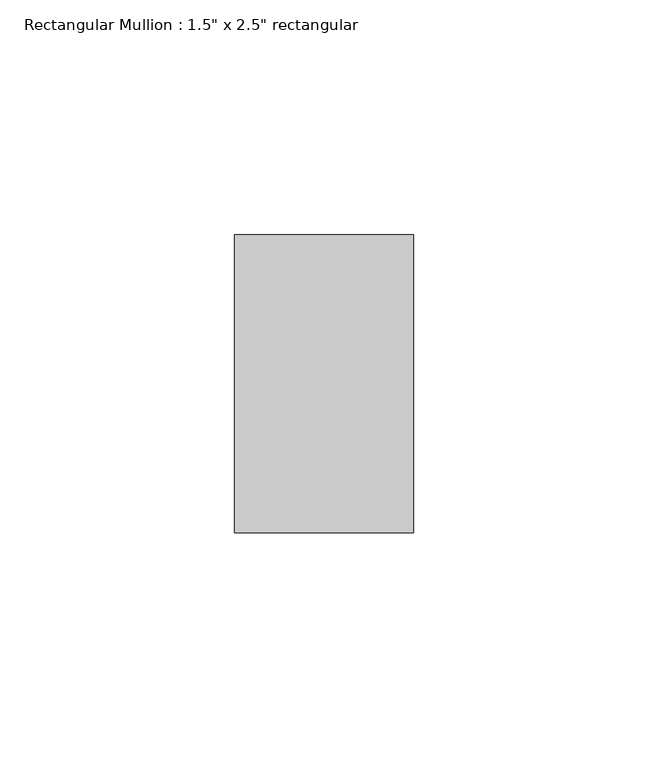
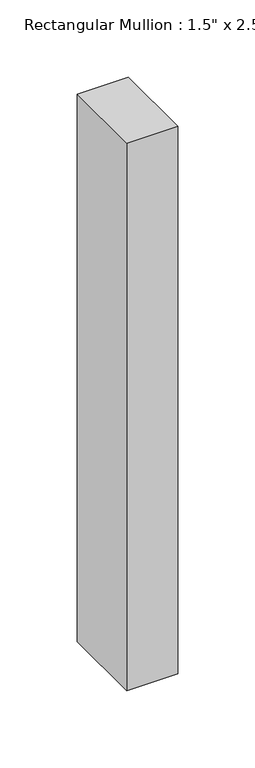
"""IFC4 building model written with IfcOpenShell, lengths in millimetres: member geometry."""

from ifc_helpers import new_model, si_unit, frame, origin, place, context, project, spatial, polyline, outline, extrude, source, transform, mapped, element, save


def member_65702978(model_context):
    return source(origin(), model_context, "Body", "SweptSolid", [
        extrude(outline(polyline([(0.0, 31.75), (0.0, -31.75), (-38.1, -31.75), (-38.1, 31.75), (0.0, 31.75)])), frame((0.0, 0.0, -431.8), z_axis=(0.0, 0.0, 1.0), x_axis=(1.0, 0.0, 0.0)), (0.0, 0.0, 1.0), 431.8),
    ])


if __name__ == "__main__":
    model = new_model("IFC4")
    model_context = context("Model", 3, world=origin())
    ifc_project = project(units=[si_unit("LENGTHUNIT", "METRE", prefix="MILLI")], contexts=[model_context])
    site = spatial("IfcSite", under=ifc_project)
    building = spatial("IfcBuilding", under=site)
    placement = place(None, origin())
    member_shape = member_65702978(model_context)
    element("IfcMember", 1, ObjectType="Rectangular Mullion : 1.5\" x 2.5\" rectangular", at=placement, inside=building, context=model_context, shape_type="MappedRepresentation", body=[
        mapped(member_shape, transform((0.0, 0.0, 0.0), x_axis=(1.0, 0.0, 0.0), y_axis=(0.0, 1.0, 0.0), z_axis=(0.0, 0.0, 1.0))),
    ])
    save(model, "model.ifc")

# Revit data of these elements
# Type "Rectangular Mullion : 1.5\" x 2.5\" rectangular"
#   built-in parameter 1007304 = 0.208333 (stored number, unit not read)
#   built-in parameter 1007301 = 0.0625 (stored number, unit not read)
#   built-in parameter 1007300 = 0.0625 (stored number, unit not read)
# Element 1 (IfcMember, "Rectangular Mullion : 1.5\" x 2.5\" rectangular")
#   Materials on its faces: "Aluminum"
# Materials
#   "Aluminum": class "Metal", colour RGB 247 247 247, transparency 0, Description = "Aluminum 6061", Cost = 0
